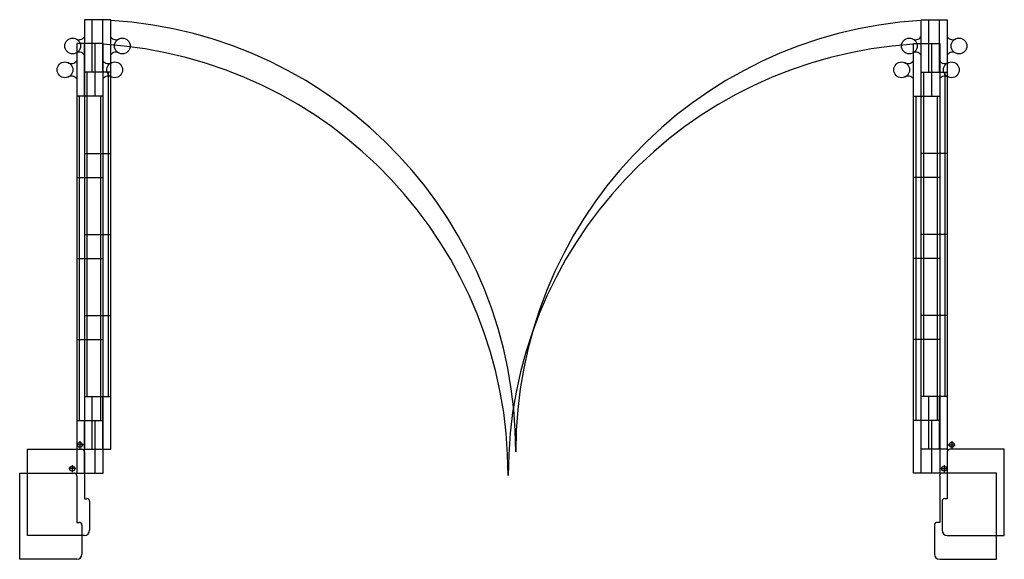
# Model space of a CAD drawing. Units: inches. Extents: x -43 to 8979, y -615 to 8149.
# Tile 5 of 5: x 313 to 1682, y 7399 to 8149. Entities that reach past the tile are written whole.
import ezdxf

# ---------------------------------------------------------------- set-up
doc = ezdxf.new("R2010")
doc.units = ezdxf.units.IN
doc.layers.add('A-DOOR', color=4, linetype='Continuous', lineweight=25)

# ---------------------------------------------------------------- blocks, each defined once
blk = doc.blocks.new('A$C0D315CAB')
for p, q in [((79.3, 717.3), (79.3, 120)), ((115.9, 717.3), (79.3, 717.3)), ((90.2, 644.2), (90.2, 717.3)), ((104.9, 644.2), (104.9, 717.3)), ((115.9, 120), (115.9, 717.3)), ((1242.7, 120), (1242.7, 717.3)), ((1242.7, 717.3), (1279.3, 717.3)), ((1253.7, 644.2), (1253.7, 717.3)), ((1268.3, 644.2), (1268.3, 717.3)), ((1279.3, 717.3), (1279.3, 120)), ((115.9, 644.2), (79.3, 644.2)), ((82.9, 644.2), (82.9, 193.2)), ((112.2, 644.2), (112.2, 193.2)), ((1242.7, 644.2), (1279.3, 644.2)), ((1246.3, 644.2), (1246.3, 193.2)), ((1275.6, 644.2), (1275.6, 193.2)), ((79.3, 531.2), (115.9, 531.2)), ((1279.3, 531.2), (1242.7, 531.2)), ((79.3, 418.5), (115.9, 418.5)), ((1279.3, 418.5), (1242.7, 418.5)), ((79.3, 305.9), (115.9, 305.9)), ((1279.3, 305.9), (1242.7, 305.9)), ((79.3, 193.2), (115.9, 193.2)), ((90.2, 120), (90.2, 193.2)), ((104.9, 120), (104.9, 193.2)), ((1279.3, 193.2), (1242.7, 193.2)), ((1253.7, 120), (1253.7, 193.2)), ((1268.3, 120), (1268.3, 193.2)), ((78.1, 126.1), (68.2, 126.1)), ((73.1, 131.1), (73.1, 121.1)), ((1280.4, 126.1), (1290.4, 126.1)), ((1285.4, 131.1), (1285.4, 121.1)), ((0, 120), (75.6, 120)), ((0, 0), (0, 120)), ((79.3, 120), (78.2, 118.9)), ((79.3, 120), (115.9, 120)), ((79.3, 116.3), (79.3, 51.2)), ((680.3, 120), (678.3, 120)), ((680.3, 120), (678.3, 120)), ((680.3, 120), (678.3, 120)), ((1279.3, 120), (1242.7, 120)), ((1279.3, 120), (1280.3, 118.9)), ((1279.3, 116.3), (1279.3, 51.2)), ((1358.5, 120), (1282.9, 120)), ((1358.5, 0), (1358.5, 120)), ((79.3, 51.2), (82.9, 51.2)), ((86.6, 47.6), (86.6, 7.3)), ((1271.9, 47.6), (1271.9, 7.3)), ((1279.3, 51.2), (1275.6, 51.2)), ((79.3, 0), (0, 0)), ((1279.3, 0), (1358.5, 0))]:
    blk.add_line(p, q)
for centre, radius in [((63, 680.8), 11), ((132.1, 680.8), 11), ((1226.4, 680.8), 11), ((1295.5, 680.8), 11), ((73.1, 126.1), 3.45), ((1285.4, 126.1), 3.45)]:
    blk.add_circle(centre, radius)
for centre, radius, start, end in [((79.6, 117.7), 599.6, 359.8723, 86.5433), ((1278.9, 117.7), 599.6, 93.4567, 180.1277), ((72, 698.2), 8.75, 234.97, 326.2886), ((123.1, 698.2), 8.75, 213.7114, 305.03), ((1235.4, 698.2), 8.75, 234.97, 326.2886), ((1286.5, 698.2), 8.75, 213.7114, 305.03), ((72, 663.4), 8.75, 33.7114, 125.03), ((123.1, 663.4), 8.75, 54.97, 146.2886), ((1235.4, 663.4), 8.75, 33.7114, 125.03), ((1286.5, 663.4), 8.75, 54.97, 146.2886), ((75.6, 116.3), 3.66, 0, 90), ((1282.9, 116.3), 3.66, 90, 180), ((82.9, 47.6), 3.66, 0, 90), ((1275.6, 47.6), 3.66, 90, 180), ((79.3, 7.3), 7.32, 270, 0), ((1279.3, 7.3), 7.32, 180, 270)]:
    blk.add_arc(centre, radius, start, end)

msp = doc.modelspace()

# ---------------------------------------------------------------- block references
at = {"layer": 'A-DOOR'}
for p in [(323.844, 7431.926), (313.194, 7398.786)]:
    msp.add_blockref('A$C0D315CAB', p, dxfattribs=at)

doc.saveas('drawing.dxf')
